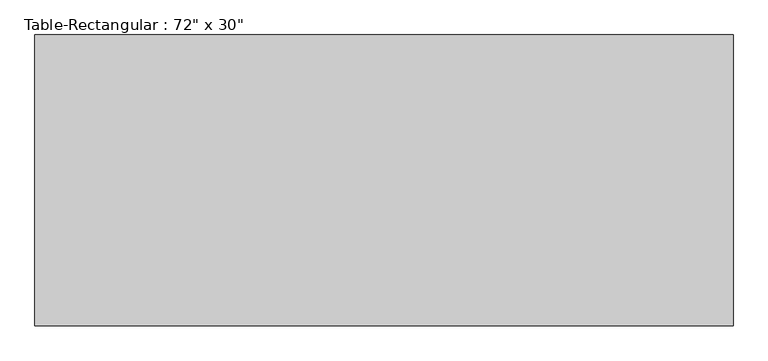
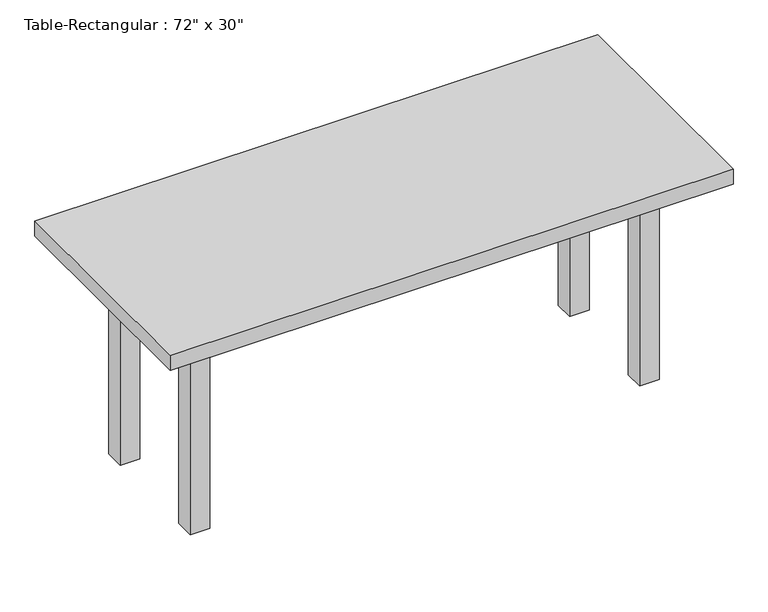
"""IFC4 building model written with IfcOpenShell, lengths in millimetres: furniture geometry."""

from ifc_helpers import new_model, si_unit, frame, origin, origin_with_axes, place, context, project, spatial, polyline, outline, extrude, source, transform, mapped, element, save


def furniture_a5b052b6(model_context):
    return source(origin(), model_context, "Body", "SweptSolid", [
        extrude(outline(polyline([(698.5, 190.5), (698.5, 165.1), (-698.5, 165.1), (-698.5, 190.5), (698.5, 190.5)])), frame((0.0, 0.0, 609.6), z_axis=(0.0, 0.0, 1.0), x_axis=(1.0, 0.0, 0.0)), (0.0, 0.0, 1.0), 101.6),
        extrude(outline(polyline([(698.5, -190.5), (-698.5, -190.5), (-698.5, -165.1), (698.5, -165.1), (698.5, -190.5)])), frame((0.0, 0.0, 609.6), z_axis=(0.0, 0.0, 1.0), x_axis=(1.0, 0.0, 0.0)), (0.0, 0.0, 1.0), 101.6),
        extrude(outline(polyline([(-711.2, -165.1), (-736.6, -165.1), (-736.6, 165.1), (-711.2, 165.1), (-711.2, -165.1)])), frame((0.0, 0.0, 609.6), z_axis=(0.0, 0.0, 1.0), x_axis=(1.0, 0.0, 0.0)), (0.0, 0.0, 1.0), 101.6),
        extrude(outline(polyline([(711.2, -165.1), (711.2, 165.1), (736.6, 165.1), (736.6, -165.1), (711.2, -165.1)])), frame((0.0, 0.0, 609.6), z_axis=(0.0, 0.0, 1.0), x_axis=(1.0, 0.0, 0.0)), (0.0, 0.0, 1.0), 101.6),
        extrude(outline(polyline([(914.4, 381.0), (914.4, -381.0), (-914.4, -381.0), (-914.4, 381.0), (914.4, 381.0)])), frame((0.0, 0.0, 711.2), z_axis=(0.0, 0.0, 1.0), x_axis=(1.0, 0.0, 0.0)), (0.0, 0.0, 1.0), 50.8),
        extrude(outline(polyline([(-698.5, 228.6), (-698.5, 165.1), (-762.0, 165.1), (-762.0, 228.6), (-698.5, 228.6)])), origin_with_axes(), (0.0, 0.0, 1.0), 711.2),
        extrude(outline(polyline([(698.5, 228.6), (762.0, 228.6), (762.0, 165.1), (698.5, 165.1), (698.5, 228.6)])), origin_with_axes(), (0.0, 0.0, 1.0), 711.2),
        extrude(outline(polyline([(-698.5, -228.6), (-762.0, -228.6), (-762.0, -165.1), (-698.5, -165.1), (-698.5, -228.6)])), origin_with_axes(), (0.0, 0.0, 1.0), 711.2),
        extrude(outline(polyline([(698.5, -228.6), (698.5, -165.1), (762.0, -165.1), (762.0, -228.6), (698.5, -228.6)])), origin_with_axes(), (0.0, 0.0, 1.0), 711.2),
    ])


if __name__ == "__main__":
    model = new_model("IFC4")
    model_context = context("Model", 3, world=origin())
    ifc_project = project(units=[si_unit("LENGTHUNIT", "METRE", prefix="MILLI")], contexts=[model_context])
    site = spatial("IfcSite", under=ifc_project)
    building = spatial("IfcBuilding", under=site)
    placement = place(None, origin())
    furniture_shape = furniture_a5b052b6(model_context)
    element("IfcFurniture", 1, ObjectType="Table-Rectangular : 72\" x 30\"", at=placement, inside=building, context=model_context, shape_type="MappedRepresentation", body=[
        mapped(furniture_shape, transform((0.0, 0.0, 0.0), x_axis=(1.0, 0.0, 0.0), y_axis=(0.0, 1.0, 0.0), z_axis=(0.0, 0.0, 1.0))),
    ])
    save(model, "model.ifc")

# Revit data of these elements
# Type "Table-Rectangular : 72\" x 30\""
#   Assembly Code = "E2020200"
#   Height = 2' - 6"
#   Length = 6' - 0"
#   Width = 2' - 6"
#   Base Material = Birch
#   Top Material = Birch
#   Default Elevation = 0
# Element 1 (IfcFurniture, "Table-Rectangular : 72\" x 30\"")
#   Materials on its faces: "Birch"
# Materials
#   "Birch": class "Wood", colour RGB 224 178 126, transparency 0, Description = "Betula Alleghaniensis", Cost = 0
